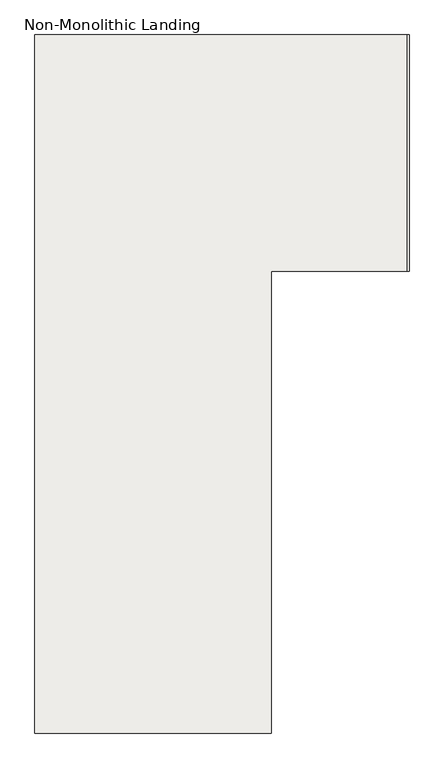
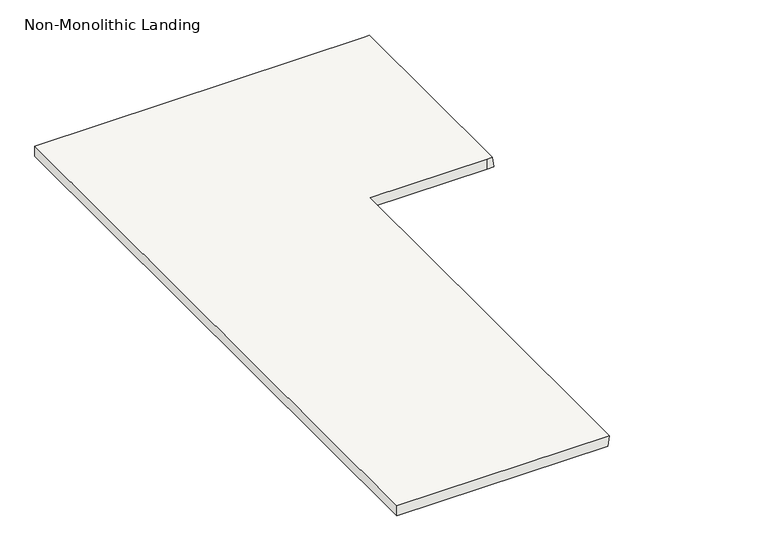
"""IFC4 building model written with IfcOpenShell, lengths in millimetres: slab geometry, Non-Monolithic Landing."""

from ifc_helpers import new_model, si_unit, origin, place, context, project, spatial, faceted_brep, source, transform, mapped, element, save


def non_monolithic_landing_d31418c5(model_context):
    return source(origin(), model_context, "Body", "Brep", [
        faceted_brep([(-11389.1151057, 2800.1398477, 1043.4782609), (-11381.9276057, 2800.1398477, 993.4782609), (-11381.9276057, 3800.1656289, 993.4782609), (-11389.1151057, 3800.1656289, 1043.4782609), (-11964.1151057, 1847.9055917, 1043.4782609), (-11964.1151057, 2800.1398477, 1043.4782609), (-11414.1151057, 2800.1398477, 1043.4782609), (-11414.1151057, 3800.1656289, 1043.4782609), (-12964.140887, 3800.1656289, 1043.4782609), (-12964.140887, 847.8798105, 1043.4782609), (-11964.1151057, 847.8798105, 1043.4782609), (-11964.1151057, 2800.1398477, 993.4782609), (-11964.1151057, 1847.9055917, 993.4782609), (-11971.3026057, 1847.9055917, 993.4782609), (-11971.3026057, 847.8798105, 993.4782609), (-12964.140887, 847.8798105, 993.4782609), (-12964.140887, 3800.1656289, 993.4782609), (-11414.1151057, 3800.1656289, 993.4782609), (-11414.1151057, 2800.1398477, 993.4782609)], [[[0, 1, 2, 3]], [[4, 5, 6, 0, 3, 7, 8, 9, 10]], [[11, 12, 13, 14, 15, 16, 17, 2, 1, 18]], [[5, 4, 12, 11]], [[6, 5, 11, 18]], [[0, 6, 18, 1]], [[7, 3, 2, 17]], [[8, 7, 17, 16]], [[9, 8, 16, 15]], [[10, 9, 15, 14]], [[4, 13, 12]], [[13, 4, 10, 14]]]),
    ])


if __name__ == "__main__":
    model = new_model("IFC4")
    model_context = context("Model", 3, world=origin())
    ifc_project = project(units=[si_unit("LENGTHUNIT", "METRE", prefix="MILLI")], contexts=[model_context])
    site = spatial("IfcSite", under=ifc_project)
    building = spatial("IfcBuilding", under=site)
    placement = place(None, origin())
    non_monolithic_landing_shape = non_monolithic_landing_d31418c5(model_context)
    element("IfcSlab", 1, ObjectType="Non-Monolithic Landing", at=placement, inside=building, context=model_context, shape_type="MappedRepresentation", body=[
        mapped(non_monolithic_landing_shape, transform((0.0, 0.0, 0.0), x_axis=(1.0, 0.0, 0.0), y_axis=(0.0, 1.0, 0.0), z_axis=(0.0, 0.0, 1.0))),
    ])
    save(model, "model.ifc")
